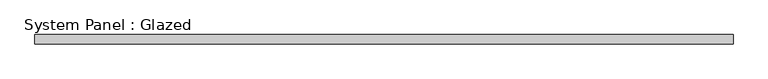
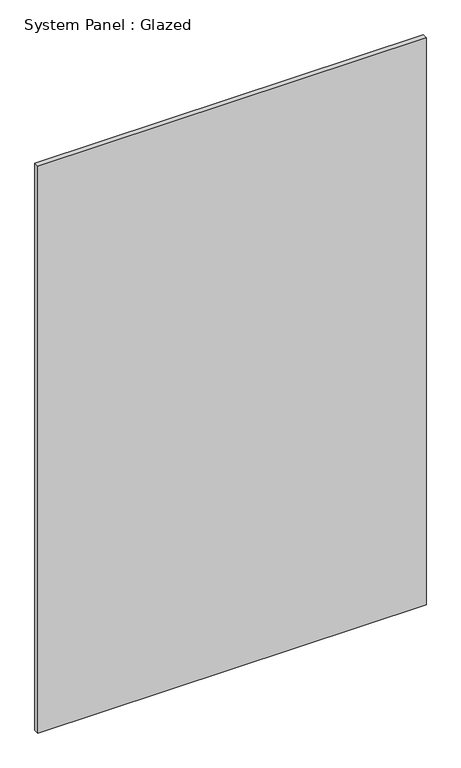
"""IFC4 building model written with IfcOpenShell, lengths in millimetres: plate geometry, System Panel : Glazed."""

from ifc_helpers import new_model, si_unit, origin, origin_with_axes, place, context, project, spatial, polyline, outline, extrude, source, transform, mapped, element, save


def system_panel_glazed_c6a8e7fc(model_context):
    return source(origin(), model_context, "Body", "SweptSolid", [
        extrude(outline(polyline([(946.1555314, 19.05), (-946.1555314, 19.05), (-946.1555314, 44.45), (946.1555314, 44.45), (946.1555314, 19.05)])), origin_with_axes(), (0.0, 0.0, 1.0), 2921.0),
    ])


if __name__ == "__main__":
    model = new_model("IFC4")
    model_context = context("Model", 3, world=origin())
    ifc_project = project(units=[si_unit("LENGTHUNIT", "METRE", prefix="MILLI")], contexts=[model_context])
    site = spatial("IfcSite", under=ifc_project)
    building = spatial("IfcBuilding", under=site)
    placement = place(None, origin())
    system_panel_glazed_shape = system_panel_glazed_c6a8e7fc(model_context)
    element("IfcPlate", 1, ObjectType="System Panel : Glazed", at=placement, inside=building, context=model_context, shape_type="MappedRepresentation", body=[
        mapped(system_panel_glazed_shape, transform((0.0, 0.0, 0.0), x_axis=(1.0, 0.0, 0.0), y_axis=(0.0, 1.0, 0.0), z_axis=(0.0, 0.0, 1.0))),
    ])
    save(model, "model.ifc")

# Revit data of these elements
# Type "System Panel : Glazed"
#   Construction Type Id = "GSP4R"
#   Analytic Construction = "1/8 in Pilkington single glazing"
#   Visual Light Transmittance = 0.9
#   Solar Heat Gain Coefficient = 0.86
#   Heat Transfer Coefficient (U) = 1.18115 BTU/(h·ft²·°F)
# Element 1 (IfcPlate, "System Panel : Glazed")
#   Materials on its faces: "Glass"
# Materials
#   "Glass": class "Glass", colour RGB 0 128 192, transparency 0.75, Description = "Soda Lime Glass", Cost = 0
